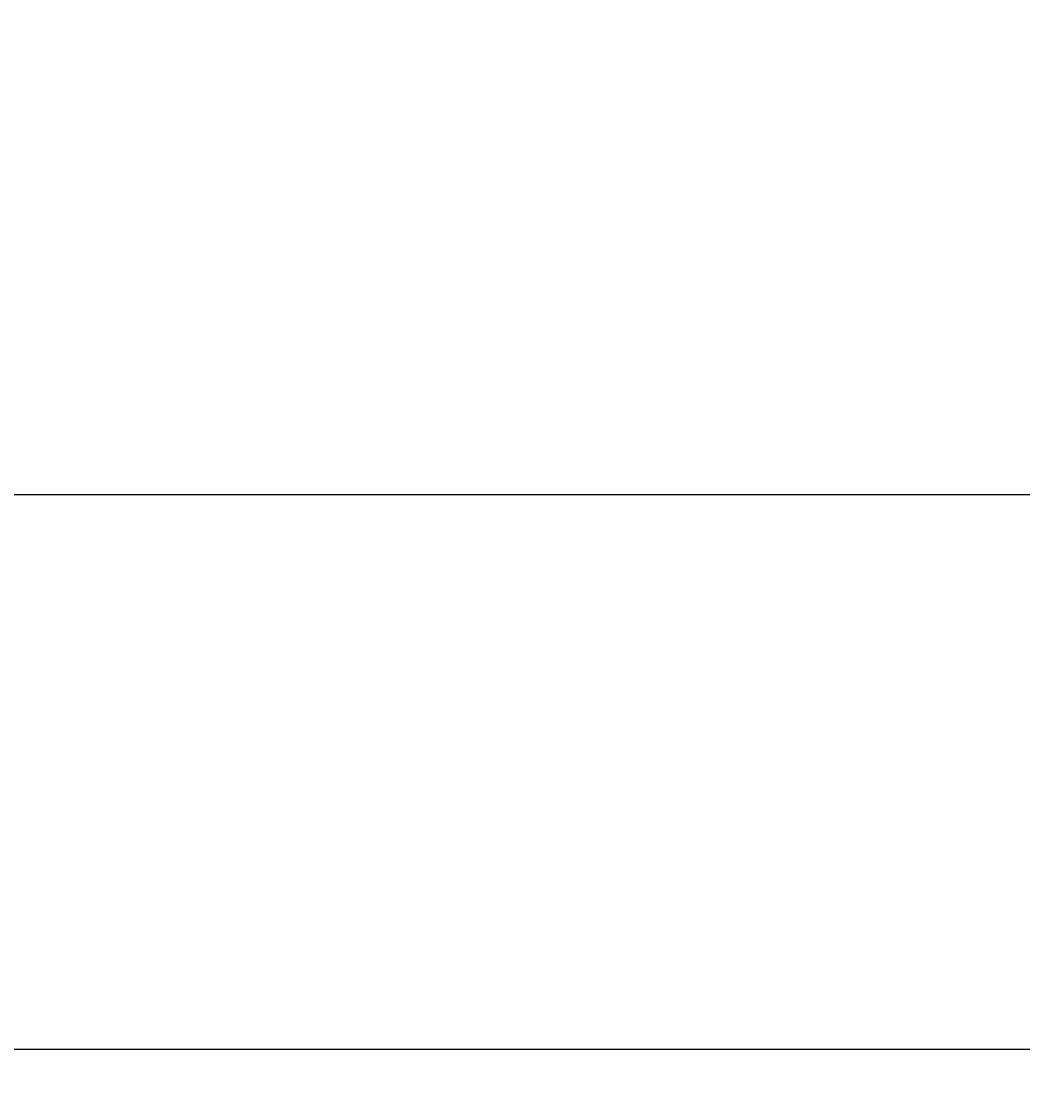
# Model space of a CAD drawing. Units: inches. Extents: x 35362 to 73946, y 43607 to 67532.
# Tile 48 of 134: x 48533 to 49302, y 46091 to 46919. Entities that reach past the tile are written whole.
import ezdxf

# ---------------------------------------------------------------- set-up
doc = ezdxf.new("R2010")
doc.units = ezdxf.units.IN
doc.header["$MEASUREMENT"] = 0
doc.layers.add('A-ANNO-DIMS', color=2, linetype='Continuous', lineweight=18)
doc.styles.get("Standard").update_dxf_attribs({"font": 'arial.ttf'})
doc.dimstyles.get("Standard").update_dxf_attribs({"dimtxt": 0.18, "dimasz": 0.18, "dimexe": 0.18, "dimexo": 0.0625, "dimgap": 0.09, "dimtad": 0, "dimtih": 1, "dimtoh": 1, "dimdec": 4, "dimzin": 0, "dimdsep": 46, "dimtxsty": 'Standard', "dimcen": 0.09, "dimadec": 0, "dimazin": 0, "dimtfac": 1, "dimtdec": 4, "dimtofl": 0, "dimtmove": 0, "dimatfit": 3, "dimfxl": 1, "dimtolj": 1, "dimtzin": 0, "dimarcsym": 0})

# ---------------------------------------------------------------- blocks, each defined once
blk = doc.blocks.new('*D5')
at = {"layer": 'A-ANNO-DIMS', "color": 0, "lineweight": -2, "transparency": 16777216}
for p, q in [((37121.95, 46919.32), (37121.95, 43606.68)), ((69871.5, 45449.83), (69871.5, 43606.68)), ((37122.13, 43606.86), (53496.29, 43606.86)), ((69871.32, 43606.86), (53497.15, 43606.86))]:
    blk.add_line(p, q, dxfattribs=at)
at = {"layer": 'A-ANNO-DIMS', "color": 0, "transparency": 16777216}
for points in [[(37122.13, 43606.89), (37122.13, 43606.83), (37121.95, 43606.86)], [(69871.32, 43606.89), (69871.32, 43606.83), (69871.5, 43606.86)]]:
    blk.add_solid(points, dxfattribs=at)
at = {"layer": 'Defpoints', "color": 0, "transparency": 16777216}
for p in [(37121.95, 46919.38), (69871.5, 45449.89), (69871.5, 43606.86)]:
    blk.add_point(p, dxfattribs=at)
at = {"layer": 'A-ANNO-DIMS', "color": 0, "transparency": 16777216, "insert": (53496.72, 43606.86), "char_height": 0.18, "attachment_point": 5}
blk.add_mtext('\\A1;32750', dxfattribs=at)
blk = doc.blocks.new('*D11')
at = {"layer": 'A-ANNO-DIMS', "color": 0, "lineweight": -2, "transparency": 16777216}
for p, q in [((47978.66, 56028.77), (47978.66, 43606.68)), ((53109.76, 56028.77), (53109.76, 43606.68)), ((47978.84, 43606.86), (50543.87, 43606.86)), ((53109.58, 43606.86), (50544.55, 43606.86))]:
    blk.add_line(p, q, dxfattribs=at)
at = {"layer": 'A-ANNO-DIMS', "color": 0, "transparency": 16777216}
for points in [[(47978.84, 43606.89), (47978.84, 43606.83), (47978.66, 43606.86)], [(53109.58, 43606.89), (53109.58, 43606.83), (53109.76, 43606.86)]]:
    blk.add_solid(points, dxfattribs=at)
at = {"layer": 'Defpoints', "color": 0, "transparency": 16777216}
for p in [(47978.66, 56028.84), (53109.76, 56028.84), (53109.76, 43606.86)]:
    blk.add_point(p, dxfattribs=at)
at = {"layer": 'A-ANNO-DIMS', "color": 0, "transparency": 16777216, "insert": (50544.21, 43606.86), "char_height": 0.18, "attachment_point": 5}
blk.add_mtext('\\A1;5131', dxfattribs=at)
blk = doc.blocks.new('*D13')
at = {"layer": 'A-ANNO-DIMS', "color": 0, "lineweight": -2, "transparency": 16777216}
for p, q in [((48373.49, 51694.02), (48373.49, 43606.68)), ((51029.04, 51694.02), (51029.04, 43606.68)), ((48373.67, 43606.86), (49700.8, 43606.86)), ((51028.86, 43606.86), (49701.73, 43606.86))]:
    blk.add_line(p, q, dxfattribs=at)
at = {"layer": 'A-ANNO-DIMS', "color": 0, "transparency": 16777216}
for points in [[(48373.67, 43606.89), (48373.67, 43606.83), (48373.49, 43606.86)], [(51028.86, 43606.89), (51028.86, 43606.83), (51029.04, 43606.86)]]:
    blk.add_solid(points, dxfattribs=at)
at = {"layer": 'Defpoints', "color": 0, "transparency": 16777216}
for p in [(48373.49, 51694.09), (51029.04, 51694.09), (51029.04, 43606.86)]:
    blk.add_point(p, dxfattribs=at)
at = {"layer": 'A-ANNO-DIMS', "color": 0, "transparency": 16777216, "insert": (49701.27, 43606.86), "char_height": 0.18, "attachment_point": 5}
blk.add_mtext('\\A1;2655.6', dxfattribs=at)
blk = doc.blocks.new('*D67')
at = {"layer": 'A-ANNO-DIMS', "color": 0, "lineweight": -2, "transparency": 16777216}
for p, q in [((56873.54, 53351.53), (35361.77, 53351.53)), ((35361.95, 53351.35), (35361.95, 49400.89)), ((35361.95, 45450.07), (35361.95, 49400.53)), ((53793.58, 45449.89), (35361.77, 45449.89))]:
    blk.add_line(p, q, dxfattribs=at)
at = {"layer": 'A-ANNO-DIMS', "color": 0, "transparency": 16777216}
for points in [[(35361.92, 53351.35), (35361.98, 53351.35), (35361.95, 53351.53)], [(35361.92, 45450.07), (35361.98, 45450.07), (35361.95, 45449.89)]]:
    blk.add_solid(points, dxfattribs=at)
at = {"layer": 'Defpoints', "color": 0, "transparency": 16777216}
for p in [(35361.95, 53351.53), (56873.6, 53351.53), (53793.64, 45449.89)]:
    blk.add_point(p, dxfattribs=at)
at = {"layer": 'A-ANNO-DIMS', "color": 0, "transparency": 16777216, "insert": (35361.95, 49400.71), "char_height": 0.18, "attachment_point": 5}
blk.add_mtext('\\A1;7901.6', dxfattribs=at)
blk = doc.blocks.new('*D76')
at = {"layer": 'A-ANNO-DIMS', "color": 0, "lineweight": -2, "transparency": 16777216}
for p, q in [((54052.84, 46555.29), (35361.77, 46555.29)), ((35361.95, 46555.11), (35361.95, 46342.27)), ((35361.95, 46129.06), (35361.95, 46341.9)), ((53793.58, 46128.88), (35361.77, 46128.88))]:
    blk.add_line(p, q, dxfattribs=at)
at = {"layer": 'A-ANNO-DIMS', "color": 0, "transparency": 16777216}
for points in [[(35361.92, 46555.11), (35361.98, 46555.11), (35361.95, 46555.29)], [(35361.92, 46129.06), (35361.98, 46129.06), (35361.95, 46128.88)]]:
    blk.add_solid(points, dxfattribs=at)
at = {"layer": 'Defpoints', "color": 0, "transparency": 16777216}
for p in [(35361.95, 46555.29), (54052.9, 46555.29), (53793.64, 46128.88)]:
    blk.add_point(p, dxfattribs=at)
at = {"layer": 'A-ANNO-DIMS', "color": 0, "transparency": 16777216, "insert": (35361.95, 46342.09), "char_height": 0.18, "attachment_point": 5}
blk.add_mtext('\\A1;426.4', dxfattribs=at)
blk = doc.blocks.new('*D90')
at = {"layer": 'A-ANNO-DIMS', "color": 0, "lineweight": -2, "transparency": 16777216}
for p, q in [((53707.72, 47291.29), (35361.77, 47291.29)), ((35361.95, 47291.11), (35361.95, 46710.26)), ((35361.95, 46129.06), (35361.95, 46709.9)), ((53793.58, 46128.88), (35361.77, 46128.88))]:
    blk.add_line(p, q, dxfattribs=at)
at = {"layer": 'A-ANNO-DIMS', "color": 0, "transparency": 16777216}
for points in [[(35361.92, 47291.11), (35361.98, 47291.11), (35361.95, 47291.29)], [(35361.92, 46129.06), (35361.98, 46129.06), (35361.95, 46128.88)]]:
    blk.add_solid(points, dxfattribs=at)
at = {"layer": 'Defpoints', "color": 0, "transparency": 16777216}
for p in [(53707.78, 47291.29), (35361.95, 46128.88), (53793.64, 46128.88)]:
    blk.add_point(p, dxfattribs=at)
at = {"layer": 'A-ANNO-DIMS', "color": 0, "transparency": 16777216, "insert": (35361.95, 46710.08), "char_height": 0.18, "attachment_point": 5}
blk.add_mtext('\\A1;1162.4', dxfattribs=at)

msp = doc.modelspace()

# ---------------------------------------------------------------- dimensions: what is measured, and where the dimension line sits
at = {"layer": 'A-ANNO-DIMS'}
for base, p1, p2, override, picture, middle in [((53109.76, 43606.859), (47978.665, 56028.836), (53109.76, 56028.836), {"dimdec": 0, "dimlfac": 1, "dimrnd": 0, "dimzin": 0, "dimdsep": 46, "dimlunit": 2}, '*D11', (50544.212, 43606.859)), ((51029.043, 43606.859), (48373.492, 51694.087), (51029.043, 51694.087), {"dimdec": 1, "dimlfac": 1, "dimrnd": 0, "dimzin": 0, "dimdsep": 46, "dimlunit": 2}, '*D13', (49701.267, 43606.859)), ((69871.496, 43606.859), (37121.949, 46919.381), (69871.496, 45449.894), {"dimdec": 0, "dimlfac": 1, "dimrnd": 0, "dimzin": 0, "dimdsep": 46, "dimlunit": 2}, '*D5', (53496.723, 43606.859))]:
    dim = msp.add_linear_dim(base=base, p1=p1, p2=p2, dimstyle='Standard', override=override, dxfattribs=at)
    dim.commit()
    dim.dimension.update_dxf_attribs({"geometry": picture, "text_midpoint": middle})
for base, p1, p2, picture, middle in [((35361.949, 53351.529), (53793.638, 45449.894), (56873.602, 53351.529), '*D67', (35361.949, 49400.712)), ((35361.949, 46128.878), (53707.781, 47291.285), (53793.638, 46128.878), '*D90', (35361.949, 46710.081)), ((35361.949, 46555.293), (53793.638, 46128.878), (54052.899, 46555.293), '*D76', (35361.949, 46342.086))]:
    dim = msp.add_linear_dim(base=base, p1=p1, p2=p2, angle=90, dimstyle='Standard', override={"dimdec": 1, "dimlfac": 1, "dimrnd": 0, "dimzin": 0, "dimdsep": 46, "dimlunit": 2}, dxfattribs=at)
    dim.commit()
    dim.dimension.update_dxf_attribs({"geometry": picture, "text_midpoint": middle})

doc.saveas('drawing.dxf')
